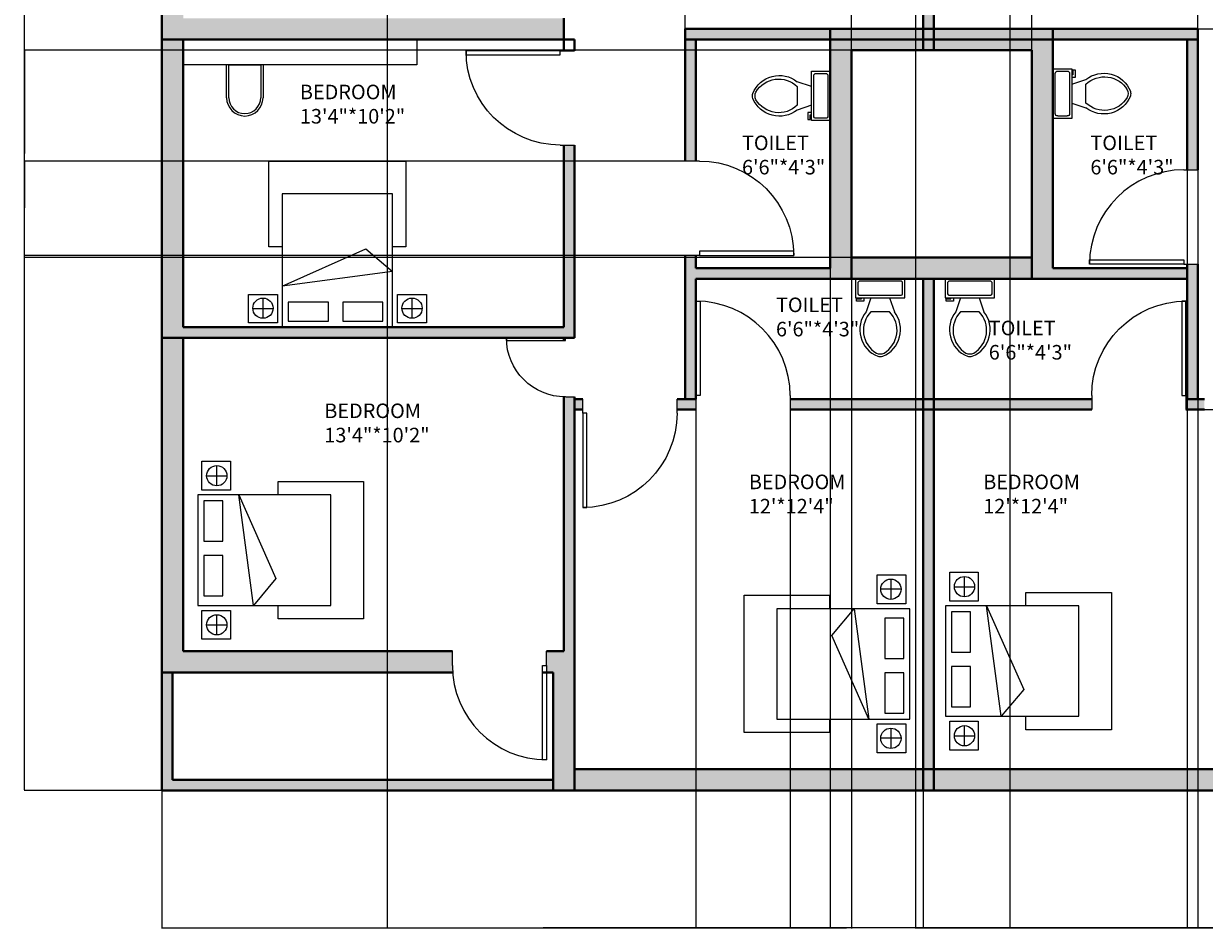
# Model space of a CAD drawing. Units: inches. Extents: x 1642 to 2399, y 1011 to 2291.
# Tile 1 of 7: x 1642 to 2143, y 1011 to 1395. Entities that reach past the tile are written whole.
import ezdxf

# ---------------------------------------------------------------- set-up
doc = ezdxf.new("R2010")
doc.units = ezdxf.units.IN
for name, color, linetype, lineweight in [('A-ANNO-DIMS', 2, 'Continuous', 18), ('A-AREA-IDEN', 7, 'Continuous', 20), ('A-DOOR', 4, 'Continuous', 25), ('A-FLOR-FIXT', 9, 'Continuous', 18), ('A-FURN', 8, 'Continuous', 18), ('A-WALL-PATT', 40, 'Continuous', 13), ('BED', 200, 'Continuous', 18), ('WALL', 40, 'Continuous', 40)]:
    doc.layers.add(name, color=color, linetype=linetype, lineweight=lineweight)
doc.styles.get("Standard").update_dxf_attribs({"font": 'arial.ttf'})
doc.dimstyles.get("Standard").update_dxf_attribs({"dimtxt": 0.18, "dimasz": 0.18, "dimexe": 0.18, "dimexo": 0.0625, "dimgap": 0.09, "dimtad": 0, "dimtih": 1, "dimtoh": 1, "dimdec": 4, "dimzin": 0, "dimdsep": 46, "dimtxsty": 'Standard', "dimcen": 0.09, "dimadec": 0, "dimazin": 0, "dimtfac": 1, "dimtdec": 4, "dimtofl": 0, "dimtmove": 0, "dimatfit": 3, "dimfxl": 1, "dimtolj": 1, "dimtzin": 0, "dimarcsym": 0})

# ---------------------------------------------------------------- blocks, each defined once
blk = doc.blocks.new('*U2')
for p, q in [((0, 0), (0, -6)), ((40, 0), (40, -6))]:
    blk.add_line(p, q)
blk.add_lwpolyline([(0, 0), (0, 40), (1.75, 40), (1.75, 0)], close=True)
blk.add_arc((0, 0), 40, 0, 90)
blk = doc.blocks.new('*U4')
for p, q in [((9.5, -6), (9.5, -2)), ((-10, -8.5), (-8, -8.5)), ((-10, -9.5), (-10, -8.5)), ((-7, -9.5), (-10, -9.5)), ((-8, -8.5), (-8, -8)), ((-7, -8), (-7, -9.5)), ((-4, -8), (-6, -14)), ((4, -8), (6, -14)), ((4, -14), (-4, -14))]:
    blk.add_line(p, q)
blk.add_lwpolyline([(10.5, -8), (10.5, 0), (-10.5, 0), (-10.5, -8)], close=True)
for points in [[(-9.5, -2), (-9.5, -6)], [(8.5, -1), (-8.5, -1)], [(-8.5, -7), (8.5, -7)]]:
    blk.add_lwpolyline(points)
for centre, radius, start, end in [((-8.62, -1.88), 0.884, 81.8699, 188.1301), ((8.62, -1.88), 0.884, 351.8699, 98.1301), ((-8.62, -6.12), 0.884, 171.8699, 278.1301), ((8.62, -6.12), 0.884, 261.8699, 8.1301), ((3.52, -21.58), 12.17, 141.4691, 247.9714), ((4.2, -21.82), 11.33, 136.3677, 238.9468), ((-3.52, -21.58), 12.17, 292.0284, 38.5307), ((-4.2, -21.82), 11.33, 301.053, 43.6321), ((0, -27.88), 4, 245.7318, 294.2682), ((0, -29), 4, 254.8605, 285.1395)]:
    blk.add_arc(centre, radius, start, end)
blk = doc.blocks.new('BED-DOUBLE-WITH-NIGHTSTANDS')
for p, q in [((8.62, 34.13), (8.62, 70.38)), ((8.62, 70.38), (66.79, 70.38)), ((66.79, 70.38), (66.79, 34.13)), ((14.22, 34.13), (8.62, 34.13)), ((14.22, 17.36), (49.69, 33.17)), ((49.69, 33.17), (61.11, 23.59)), ((66.79, 34.13), (61.11, 34.13)), ((61.11, 23.59), (14.22, 17.36)), ((6.17, 3.76), (6.17, 12.35)), ((69.41, 3.76), (69.41, 12.35)), ((1.82, 7.94), (10.42, 7.94)), ((65.06, 7.94), (73.65, 7.94))]:
    blk.add_line(p, q)
for points in [[(14.22, 0), (61.11, 0), (61.11, 56.52), (14.22, 56.52)], [(12.24, 1.79), (0, 1.79), (0, 13.82), (12.24, 13.82)], [(16.77, 2.51), (33.87, 2.51), (33.87, 10.66), (16.77, 10.66)], [(39.94, 2.51), (57.04, 2.51), (57.04, 10.66), (39.94, 10.66)], [(75.48, 1.79), (63.24, 1.79), (63.24, 13.82), (75.48, 13.82)]]:
    blk.add_lwpolyline(points, close=True)
for centre in [(6.12, 8.05), (69.36, 8.05)]:
    blk.add_circle(centre, 4.3)
blk = doc.blocks.new('DESK-WITH-CHAIR')
blk.add_lwpolyline([(0, 32.44), (99.14, 32.44), (99.14, 21.72), (0, 21.72)], close=True)
for points in [[(18.41, 7.73), (18.41, 21.72)], [(19.41, 7.73), (19.41, 21.72), (32.87, 21.72), (32.87, 7.73)], [(33.87, 21.72), (33.87, 7.73)]]:
    blk.add_lwpolyline(points)
for radius in [7.73, 6.73]:
    blk.add_arc((26.14, 7.73), radius, 180, 0)
blk = doc.blocks.new('*D33')
at = {"layer": 'A-ANNO-DIMS', "color": 0, "lineweight": -2, "transparency": 16777216}
for p, q in [((1700.65, 2232.46), (1642.19, 2232.46)), ((1642.37, 2232.28), (1642.37, 1651.26)), ((1642.37, 1069.89), (1642.37, 1650.9)), ((1700.65, 1069.71), (1642.19, 1069.71))]:
    blk.add_line(p, q, dxfattribs=at)
at = {"layer": 'A-ANNO-DIMS', "color": 0, "transparency": 16777216}
for points in [[(1642.34, 2232.28), (1642.4, 2232.28), (1642.37, 2232.46)], [(1642.34, 1069.89), (1642.4, 1069.89), (1642.37, 1069.71)]]:
    blk.add_solid(points, dxfattribs=at)
at = {"layer": 'Defpoints', "color": 0, "transparency": 16777216}
for p in [(1642.37, 2232.46), (1700.71, 2232.46), (1700.71, 1069.71)]:
    blk.add_point(p, dxfattribs=at)
at = {"layer": 'A-ANNO-DIMS', "color": 0, "transparency": 16777216, "insert": (1642.37, 1651.08), "char_height": 0.18, "attachment_point": 5}
blk.add_mtext('\\A1;1162.7', dxfattribs=at)
blk = doc.blocks.new('*D40')
at = {"layer": 'A-ANNO-DIMS', "color": 0, "lineweight": -2, "transparency": 16777216}
for p, q in [((1796.18, 1709.39), (1796.18, 1011.19)), ((2186.88, 1709.39), (2186.88, 1011.19)), ((1796.36, 1011.37), (1991.13, 1011.37)), ((2186.7, 1011.37), (1991.92, 1011.37))]:
    blk.add_line(p, q, dxfattribs=at)
at = {"layer": 'A-ANNO-DIMS', "color": 0, "transparency": 16777216}
for points in [[(1796.36, 1011.4), (1796.36, 1011.34), (1796.18, 1011.37)], [(2186.7, 1011.4), (2186.7, 1011.34), (2186.88, 1011.37)]]:
    blk.add_solid(points, dxfattribs=at)
at = {"layer": 'Defpoints', "color": 0, "transparency": 16777216}
for p in [(1796.18, 1709.46), (2186.88, 1709.46), (2186.88, 1011.37)]:
    blk.add_point(p, dxfattribs=at)
at = {"layer": 'A-ANNO-DIMS', "color": 0, "transparency": 16777216, "insert": (1991.53, 1011.37), "char_height": 0.18, "attachment_point": 5}
blk.add_mtext('\\A1;390.7', dxfattribs=at)
blk = doc.blocks.new('*D44')
at = {"layer": 'A-ANNO-DIMS', "color": 0, "lineweight": -2, "transparency": 16777216}
for p, q in [((1700.71, 1069.65), (1700.71, 1011.19)), ((2023.71, 1069.65), (2023.71, 1011.19)), ((1700.89, 1011.37), (1861.92, 1011.37)), ((2023.53, 1011.37), (1862.5, 1011.37))]:
    blk.add_line(p, q, dxfattribs=at)
at = {"layer": 'A-ANNO-DIMS', "color": 0, "transparency": 16777216}
for points in [[(1700.89, 1011.4), (1700.89, 1011.34), (1700.71, 1011.37)], [(2023.53, 1011.4), (2023.53, 1011.34), (2023.71, 1011.37)]]:
    blk.add_solid(points, dxfattribs=at)
at = {"layer": 'Defpoints', "color": 0, "transparency": 16777216}
for p in [(1700.71, 1069.71), (2023.71, 1069.71), (2023.71, 1011.37)]:
    blk.add_point(p, dxfattribs=at)
at = {"layer": 'A-ANNO-DIMS', "color": 0, "transparency": 16777216, "insert": (1862.21, 1011.37), "char_height": 0.18, "attachment_point": 5}
blk.add_mtext('\\A1;323', dxfattribs=at)
blk = doc.blocks.new('*D45')
at = {"layer": 'A-ANNO-DIMS', "color": 0, "lineweight": -2, "transparency": 16777216}
for p, q in [((2023.71, 1069.65), (2023.71, 1011.19)), ((2340.18, 1069.65), (2340.18, 1011.19)), ((2023.89, 1011.37), (2181.55, 1011.37)), ((2340, 1011.37), (2182.34, 1011.37))]:
    blk.add_line(p, q, dxfattribs=at)
at = {"layer": 'A-ANNO-DIMS', "color": 0, "transparency": 16777216}
for points in [[(2023.89, 1011.4), (2023.89, 1011.34), (2023.71, 1011.37)], [(2340, 1011.4), (2340, 1011.34), (2340.18, 1011.37)]]:
    blk.add_solid(points, dxfattribs=at)
at = {"layer": 'Defpoints', "color": 0, "transparency": 16777216}
for p in [(2023.71, 1069.71), (2340.18, 1069.71), (2340.18, 1011.37)]:
    blk.add_point(p, dxfattribs=at)
at = {"layer": 'A-ANNO-DIMS', "color": 0, "transparency": 16777216, "insert": (2181.95, 1011.37), "char_height": 0.18, "attachment_point": 5}
blk.add_mtext('\\A1;316.5', dxfattribs=at)
blk = doc.blocks.new('*D46')
at = {"layer": 'A-ANNO-DIMS', "color": 0, "lineweight": -2, "transparency": 16777216}
for p, q in [((2020.45, 1709.39), (2020.45, 1011.19)), ((2060.45, 1709.39), (2060.45, 1011.19)), ((2020.63, 1011.37), (2040.22, 1011.37)), ((2060.27, 1011.37), (2040.67, 1011.37))]:
    blk.add_line(p, q, dxfattribs=at)
at = {"layer": 'A-ANNO-DIMS', "color": 0, "transparency": 16777216}
for points in [[(2020.63, 1011.4), (2020.63, 1011.34), (2020.45, 1011.37)], [(2060.27, 1011.4), (2060.27, 1011.34), (2060.45, 1011.37)]]:
    blk.add_solid(points, dxfattribs=at)
at = {"layer": 'Defpoints', "color": 0, "transparency": 16777216}
for p in [(2020.45, 1709.46), (2060.45, 1709.46), (2060.45, 1011.37)]:
    blk.add_point(p, dxfattribs=at)
at = {"layer": 'A-ANNO-DIMS', "color": 0, "transparency": 16777216, "insert": (2040.45, 1011.37), "char_height": 0.18, "attachment_point": 5}
blk.add_mtext('\\A1;40', dxfattribs=at)
blk = doc.blocks.new('*D48')
at = {"layer": 'A-ANNO-DIMS', "color": 0, "lineweight": -2, "transparency": 16777216}
for p, q in [((1922.74, 1392.77), (1922.74, 2290.98)), ((1922.92, 2290.8), (2031.1, 2290.8)), ((2140.06, 2290.8), (2031.89, 2290.8)), ((2140.24, 1392.77), (2140.24, 2290.98))]:
    blk.add_line(p, q, dxfattribs=at)
at = {"layer": 'A-ANNO-DIMS', "color": 0, "transparency": 16777216}
for points in [[(1922.92, 2290.83), (1922.92, 2290.77), (1922.74, 2290.8)], [(2140.06, 2290.83), (2140.06, 2290.77), (2140.24, 2290.8)]]:
    blk.add_solid(points, dxfattribs=at)
at = {"layer": 'Defpoints', "color": 0, "transparency": 16777216}
for p in [(2140.24, 2290.8), (1922.74, 1392.71), (2140.24, 1392.71)]:
    blk.add_point(p, dxfattribs=at)
at = {"layer": 'A-ANNO-DIMS', "color": 0, "transparency": 16777216, "insert": (2031.49, 2290.8), "char_height": 0.18, "attachment_point": 5}
blk.add_mtext('\\A1;217.5', dxfattribs=at)
blk = doc.blocks.new('*D49')
at = {"layer": 'A-ANNO-DIMS', "color": 0, "lineweight": -2, "transparency": 16777216}
for p, q in [((2140.3, 1392.71), (2398.73, 1392.71)), ((2398.55, 1392.53), (2398.55, 1312.16)), ((2398.55, 1231.42), (2398.55, 1311.79)), ((2135.24, 1231.24), (2398.73, 1231.24))]:
    blk.add_line(p, q, dxfattribs=at)
at = {"layer": 'A-ANNO-DIMS', "color": 0, "transparency": 16777216}
for points in [[(2398.52, 1392.53), (2398.58, 1392.53), (2398.55, 1392.71)], [(2398.52, 1231.42), (2398.58, 1231.42), (2398.55, 1231.24)]]:
    blk.add_solid(points, dxfattribs=at)
at = {"layer": 'Defpoints', "color": 0, "transparency": 16777216}
for p in [(2140.24, 1392.71), (2135.18, 1231.24), (2398.55, 1231.24)]:
    blk.add_point(p, dxfattribs=at)
at = {"layer": 'A-ANNO-DIMS', "color": 0, "transparency": 16777216, "insert": (2398.55, 1311.98), "char_height": 0.18, "attachment_point": 5}
blk.add_mtext('\\A1;161.46', dxfattribs=at)
blk = doc.blocks.new('*D50')
at = {"layer": 'A-ANNO-DIMS', "color": 0, "lineweight": -2, "transparency": 16777216}
for p, q in [((1993.24, 1295.77), (1993.24, 2290.98)), ((1993.42, 2290.8), (2031.17, 2290.8)), ((2069.56, 2290.8), (2031.82, 2290.8)), ((2069.74, 1295.77), (2069.74, 2290.98))]:
    blk.add_line(p, q, dxfattribs=at)
at = {"layer": 'A-ANNO-DIMS', "color": 0, "transparency": 16777216}
for points in [[(1993.42, 2290.83), (1993.42, 2290.77), (1993.24, 2290.8)], [(2069.56, 2290.83), (2069.56, 2290.77), (2069.74, 2290.8)]]:
    blk.add_solid(points, dxfattribs=at)
at = {"layer": 'Defpoints', "color": 0, "transparency": 16777216}
for p in [(2069.74, 2290.8), (1993.24, 1295.71), (2069.74, 1295.71)]:
    blk.add_point(p, dxfattribs=at)
at = {"layer": 'A-ANNO-DIMS', "color": 0, "transparency": 16777216, "insert": (2031.49, 2290.8), "char_height": 0.18, "attachment_point": 5}
blk.add_mtext('\\A1;76.5', dxfattribs=at)
blk = doc.blocks.new('*D51')
at = {"layer": 'A-ANNO-DIMS', "color": 0, "lineweight": -2, "transparency": 16777216}
for p, q in [((2069.68, 1383.71), (1642.19, 1383.71)), ((1642.37, 1383.53), (1642.37, 1339.89)), ((1642.37, 1295.89), (1642.37, 1339.53)), ((2069.68, 1295.71), (1642.19, 1295.71))]:
    blk.add_line(p, q, dxfattribs=at)
at = {"layer": 'A-ANNO-DIMS', "color": 0, "transparency": 16777216}
for points in [[(1642.34, 1383.53), (1642.4, 1383.53), (1642.37, 1383.71)], [(1642.34, 1295.89), (1642.4, 1295.89), (1642.37, 1295.71)]]:
    blk.add_solid(points, dxfattribs=at)
at = {"layer": 'Defpoints', "color": 0, "transparency": 16777216}
for p in [(1642.37, 1383.71), (2069.74, 1383.71), (2069.74, 1295.71)]:
    blk.add_point(p, dxfattribs=at)
at = {"layer": 'A-ANNO-DIMS', "color": 0, "transparency": 16777216, "insert": (1642.37, 1339.71), "char_height": 0.18, "attachment_point": 5}
blk.add_mtext('\\A1;88', dxfattribs=at)
blk = doc.blocks.new('*D52')
at = {"layer": 'A-ANNO-DIMS', "color": 0, "lineweight": -2, "transparency": 16777216}
for p, q in [((1922.68, 1336.67), (1642.19, 1336.67)), ((1642.37, 1336.49), (1642.37, 1316.85)), ((1642.37, 1296.85), (1642.37, 1316.49)), ((1922.68, 1296.67), (1642.19, 1296.67))]:
    blk.add_line(p, q, dxfattribs=at)
at = {"layer": 'A-ANNO-DIMS', "color": 0, "transparency": 16777216}
for points in [[(1642.34, 1336.49), (1642.4, 1336.49), (1642.37, 1336.67)], [(1642.34, 1296.85), (1642.4, 1296.85), (1642.37, 1296.67)]]:
    blk.add_solid(points, dxfattribs=at)
at = {"layer": 'Defpoints', "color": 0, "transparency": 16777216}
for p in [(1642.37, 1336.67), (1922.74, 1336.67), (1922.74, 1296.67)]:
    blk.add_point(p, dxfattribs=at)
at = {"layer": 'A-ANNO-DIMS', "color": 0, "transparency": 16777216, "insert": (1642.37, 1316.67), "char_height": 0.18, "attachment_point": 5}
blk.add_mtext('\\A1;40', dxfattribs=at)
blk = doc.blocks.new('*D53')
at = {"layer": 'A-ANNO-DIMS', "color": 0, "lineweight": -2, "transparency": 16777216}
for p, q in [((1927.24, 1235.65), (1927.24, 1011.19)), ((1967.24, 1235.65), (1967.24, 1011.19)), ((1927.42, 1011.37), (1947.02, 1011.37)), ((1967.06, 1011.37), (1947.46, 1011.37))]:
    blk.add_line(p, q, dxfattribs=at)
at = {"layer": 'A-ANNO-DIMS', "color": 0, "transparency": 16777216}
for points in [[(1927.42, 1011.4), (1927.42, 1011.34), (1927.24, 1011.37)], [(1967.06, 1011.4), (1967.06, 1011.34), (1967.24, 1011.37)]]:
    blk.add_solid(points, dxfattribs=at)
at = {"layer": 'Defpoints', "color": 0, "transparency": 16777216}
for p in [(1927.24, 1235.71), (1967.24, 1235.71), (1967.24, 1011.37)]:
    blk.add_point(p, dxfattribs=at)
at = {"layer": 'A-ANNO-DIMS', "color": 0, "transparency": 16777216, "insert": (1947.24, 1011.37), "char_height": 0.18, "attachment_point": 5}
blk.add_mtext('\\A1;40', dxfattribs=at)
blk = doc.blocks.new('*D54')
at = {"layer": 'A-ANNO-DIMS', "color": 0, "lineweight": -2, "transparency": 16777216}
for p, q in [((1984.24, 1388.15), (1984.24, 1011.19)), ((1993.24, 1383.65), (1993.24, 1011.19)), ((1984.42, 1011.37), (1988.59, 1011.37)), ((1993.06, 1011.37), (1988.89, 1011.37))]:
    blk.add_line(p, q, dxfattribs=at)
at = {"layer": 'A-ANNO-DIMS', "color": 0, "transparency": 16777216}
for points in [[(1984.42, 1011.4), (1984.42, 1011.34), (1984.24, 1011.37)], [(1993.06, 1011.4), (1993.06, 1011.34), (1993.24, 1011.37)]]:
    blk.add_solid(points, dxfattribs=at)
at = {"layer": 'Defpoints', "color": 0, "transparency": 16777216}
for p in [(1984.24, 1388.21), (1993.24, 1383.71), (1993.24, 1011.37)]:
    blk.add_point(p, dxfattribs=at)
at = {"layer": 'A-ANNO-DIMS', "color": 0, "transparency": 16777216, "insert": (1988.74, 1011.37), "char_height": 0.18, "attachment_point": 5}
blk.add_mtext('\\A1;9', dxfattribs=at)
blk = doc.blocks.new('*D55')
at = {"layer": 'A-ANNO-DIMS', "color": 0, "lineweight": -2, "transparency": 16777216}
for p, q in [((2135.74, 1388.15), (2135.74, 1011.19)), ((2140.24, 1392.65), (2140.24, 1011.19)), ((2135.92, 1011.37), (2137.73, 1011.37)), ((2140.06, 1011.37), (2138.25, 1011.37))]:
    blk.add_line(p, q, dxfattribs=at)
at = {"layer": 'A-ANNO-DIMS', "color": 0, "transparency": 16777216}
for points in [[(2135.92, 1011.4), (2135.92, 1011.34), (2135.74, 1011.37)], [(2140.06, 1011.4), (2140.06, 1011.34), (2140.24, 1011.37)]]:
    blk.add_solid(points, dxfattribs=at)
at = {"layer": 'Defpoints', "color": 0, "transparency": 16777216}
for p in [(2135.74, 1388.21), (2140.24, 1392.71), (2140.24, 1011.37)]:
    blk.add_point(p, dxfattribs=at)
at = {"layer": 'A-ANNO-DIMS', "color": 0, "transparency": 16777216, "insert": (2137.99, 1011.37), "char_height": 0.18, "attachment_point": 5}
blk.add_mtext('\\A1;4.5', dxfattribs=at)

msp = doc.modelspace()

# ---------------------------------------------------------------- hatches: boundary and pattern name
at = {"layer": 'A-WALL-PATT'}
h = msp.add_hatch(color=256, dxfattribs=at)
h.dxf.hatch_style = 1
h.paths.add_polyline_path([(2340.1804, 2185.4562), (2211.0983, 2185.4562, -0.01876983), (2211.211, 2182.4562), (2211.211, 2176.4562), (2331.211, 2176.4562), (2331.211, 2043.4562), (2171.211, 2043.4562), (2171.211, 2038.9562), (2331.211, 2038.9562), (2331.211, 1916.9562), (2171.211, 1916.9562), (2171.211, 1918.9365), (2166.711, 1918.9365), (2166.711, 1912.4562), (2340.1804, 1912.4562)])
h.paths.add_polyline_path([(2171.211, 2043.4562), (2171.211, 2043.9025), (2170.5217, 2043.9025), (2166.711, 2043.9025), (2166.711, 2038.9562), (2166.711, 1958.9365), (2171.211, 1958.9365)], flags=17)
h.paths.add_polyline_path([(2129.211, 1971.5979), (2124.711, 1971.5979), (2124.711, 1918.4562), (2067.711, 1918.4562), (2067.711, 1913.9562), (2129.211, 1913.9562)])
h.paths.add_polyline_path([(2067.711, 2015.4562), (2124.711, 2015.4562), (2124.711, 2019.9562), (2058.711, 2019.9562), (2058.711, 2015.4562), (2058.711, 1922.9562), (1982.211, 1922.9562), (1982.211, 2015.4562), (1982.211, 2019.9562), (1916.211, 2019.9562), (1916.211, 2070.9562), (1911.711, 2070.9562), (1911.711, 2015.4562), (1911.711, 2012.302), (1916.211, 2012.302), (1916.211, 2015.4562), (1973.211, 2015.4562), (1973.211, 1918.4562), (1973.211, 1913.9562), (2017.1804, 1913.9562), (2067.711, 1913.9562), (2067.711, 1918.4562)])
h.paths.add_polyline_path([(2131.1386, 2075.4562), (2118.1934, 2075.4562), (2118.1934, 2070.9562), (2131.1386, 2070.9562)], flags=17)
h.paths.add_polyline_path([(1918.8034, 2075.4562), (1909.4956, 2075.4562), (1909.4956, 2070.9562), (1918.8034, 2070.9562)], flags=17)
h.paths.add_polyline_path([(1874.211, 2029.9562), (1869.711, 2029.9562), (1869.711, 1960.7404), (1874.211, 1960.7404)], flags=17)
h.paths.add_polyline_path([(1916.211, 1972.302), (1911.711, 1972.302), (1911.711, 1918.4562), (1916.211, 1918.4562)], flags=17)
h.paths.add_polyline_path([(2340.1804, 1912.4562), (2331.1804, 1912.4562), (2331.1804, 1794.4562), (2210.1804, 1794.4562), (2210.1804, 1789.9562), (2279.6804, 1789.9562), (2340.1804, 1789.9562)])
h.paths.add_polyline_path([(2288.6804, 1789.9562), (2279.6804, 1789.9562), (2279.6804, 1785.0846), (2285.6804, 1785.0846), (2288.6804, 1785.0846)], flags=17)
h.paths.add_polyline_path([(2169.6804, 1789.9562), (2170.1804, 1789.9562), (2170.1804, 1794.4562), (2165.1804, 1794.4562), (2165.1804, 1713.9562), (2165.1804, 1709.4562), (2279.6804, 1709.4562), (2279.6804, 1718.4562), (2169.6804, 1718.4562)])
h.paths.add_polyline_path([(2288.6804, 1745.1973, -0.01876983), (2285.6804, 1745.0846), (2279.6804, 1745.0846), (2279.6804, 1709.4562), (2340.1804, 1709.4562), (2340.1804, 1789.9562), (2335.6804, 1789.9562), (2335.6804, 1713.9562), (2288.6804, 1713.9562)])
h.paths.add_polyline_path([(2165.1804, 1713.9562), (2140.6229, 1713.9562), (2088.923, 1713.9562), (2069.7509, 1713.9562), (2060.4457, 1713.9562), (2060.4457, 1709.4562), (2165.1804, 1709.4562)])
h.paths.add_polyline_path([(2020.4457, 1713.9562), (2017.1804, 1713.9562), (2012.6804, 1713.9562), (2009.1946, 1713.9562), (2009.1946, 1709.4562), (2020.4457, 1709.4562)])
h.paths.add_polyline_path([(1969.1946, 1713.9562), (1864.6804, 1713.9562), (1864.6804, 1798.9562), (1860.1804, 1798.9562), (1860.1804, 1792.9562), (1860.1804, 1752.9562), (1860.1804, 1718.4562), (1750.1804, 1718.4562), (1750.1804, 1749.2419), (1744.1804, 1749.2419, -0.01876983), (1741.1804, 1749.3546), (1741.1804, 1709.4562), (1969.1946, 1709.4562)])
h.paths.add_polyline_path([(1741.1804, 1803.4562), (1700.711, 1803.4562), (1700.711, 1794.4562), (1741.1804, 1794.4562)])
h.paths.add_polyline_path([(1820.1804, 1798.9562), (1741.1804, 1798.9562), (1741.1804, 1794.4562), (1741.1804, 1790.0365), (1741.1804, 1789.2419), (1744.1804, 1789.2419), (1750.1804, 1789.2419), (1750.1804, 1794.4562), (1820.1804, 1794.4562)], flags=17)
h.paths.add_polyline_path([(1800.6804, 1709.4562), (1796.1804, 1709.4562), (1796.1804, 1592.7078), (1978.9325, 1592.7078), (1978.9325, 1597.2078), (1800.6804, 1597.2078)])
h.paths.add_polyline_path([(2097.0678, 1709.4562), (2088.0678, 1709.4562), (2088.0678, 1599.6874), (2088.0678, 1597.2078), (2097.0678, 1597.2078)], flags=17)
h.paths.add_polyline_path([(2186.8766, 1709.4562), (2182.3766, 1709.4562), (2182.3766, 1597.2078), (2071.4624, 1597.2078), (2071.4624, 1592.7078), (2186.8766, 1592.7078)])
h.paths.add_polyline_path([(2078.1934, 2075.4562), (2022.711, 2075.4562), (2022.711, 2223.4562), (2166.711, 2223.4562), (2166.711, 2075.4562), (2166.711, 2070.9562), (2171.211, 2070.9562), (2171.211, 2138.8919), (2171.211, 2227.9562), (2335.711, 2227.9562), (2335.711, 2185.4562), (2340.1804, 2185.4562), (2340.1804, 2232.4562), (1874.211, 2232.4562), (1874.211, 2223.4562), (2018.211, 2223.4562), (2018.211, 2075.4562), (1958.8034, 2075.4562), (1958.8034, 2070.9562), (2018.211, 2070.9562), (2018.211, 2019.9562), (1982.211, 2019.9562), (1982.211, 2015.4562), (1982.211, 2010.9562), (2058.711, 2010.9562), (2058.711, 2015.4562), (2058.711, 2019.9562), (2022.711, 2019.9562), (2022.711, 2070.9562), (2078.1934, 2070.9562)])
h.paths.add_polyline_path([(1874.211, 2171.9562), (1874.211, 2176.4562), (1861.9371, 2176.4562), (1861.9371, 2173.4562), (1861.9371, 2167.4562), (1869.711, 2167.4562), (1869.711, 2069.7602), (1874.211, 2069.7602)], flags=17)
h.paths.add_polyline_path([(1705.211, 2227.9562), (1865.211, 2227.9562), (1865.211, 2176.4562), (1874.211, 2176.4562), (1874.211, 2232.4562), (1700.711, 2232.4562), (1700.711, 2176.4562), (1705.211, 2176.4562)])
h.paths.add_polyline_path([(1709.711, 2167.4562), (1821.9371, 2167.4562), (1821.9371, 2173.4562, -0.01876983), (1822.0498, 2176.4562), (1700.711, 2176.4562), (1700.711, 1913.9562), (1860.1804, 1913.9562), (1864.6804, 1913.9562), (1973.211, 1913.9562), (1973.211, 1918.4562), (1916.211, 1918.4562), (1874.211, 1918.4562), (1874.211, 1920.7404), (1869.711, 1920.7404), (1869.711, 1918.4562), (1860.1804, 1918.4562), (1709.711, 1918.4562), (1709.711, 2029.9562), (1874.211, 2029.9562), (1874.211, 2037.0364), (1869.711, 2037.0364), (1869.711, 2034.4562), (1709.711, 2034.4562)])
h.paths.add_polyline_path([(2017.1804, 1913.9562), (2012.6804, 1913.9562), (2012.6804, 1713.9562), (2017.1804, 1713.9562)])
h.paths.add_polyline_path([(1952.4341, 2110.3716), (2000.4134, 2110.3716), (2000.4134, 2133.4189), (1952.4341, 2133.4189)], flags=25)
h.paths.add_polyline_path([(2042.3983, 2110.7121), (2090.3775, 2110.7121), (2090.3775, 2133.7594), (2042.3983, 2133.7594)], flags=25)
h.paths.add_polyline_path([(2201.7332, 2091.8715), (2249.7125, 2091.8715), (2249.7125, 2114.9188), (2201.7332, 2114.9188)], flags=25)
h.paths.add_polyline_path([(1805.186, 2077.6915), (1853.1653, 2077.6915), (1853.1653, 2100.7388), (1805.186, 2100.7388)], flags=25)
h.paths.add_polyline_path([(1794.8897, 1974.6584), (1842.869, 1974.6584), (1842.869, 1997.7057), (1794.8897, 1997.7057)], flags=25)
h.paths.add_polyline_path([(2229.1796, 2204.4209), (2315.1362, 2204.4209), (2315.1362, 2217.1488), (2229.1796, 2217.1488)], flags=25)
h.paths.add_polyline_path([(1715.2159, 2199.5328), (1801.1724, 2199.5328), (1801.1724, 2212.2607), (1715.2159, 2212.2607)], flags=25)
h.paths.add_polyline_path([(2230.7681, 1755.7109), (2271.7283, 1755.7109), (2271.7283, 1778.7582), (2230.7681, 1778.7582)], flags=25)
h.paths.add_polyline_path([(1763.4713, 1764.1742), (1804.4315, 1764.1742), (1804.4315, 1787.2215), (1763.4713, 1787.2215)], flags=25)
h.paths.add_polyline_path([(2076.2643, 1955.0495), (2111.326, 1955.0495), (2111.326, 1978.0968), (2076.2643, 1978.0968)], flags=25)
h.paths.add_polyline_path([(1932.854, 1956.1217), (1967.9158, 1956.1217), (1967.9158, 1979.169), (1932.854, 1979.169)], flags=25)
h.paths.add_polyline_path([(2048.1203, 2031.6107), (2083.1821, 2031.6107), (2083.1821, 2054.658), (2048.1203, 2054.658)], flags=25)
h.paths.add_polyline_path([(2163.5754, 1863.7569), (2208.2347, 1863.7569), (2208.2347, 1886.8042), (2163.5754, 1886.8042)], flags=9)
h.paths.add_polyline_path([(2039.9286, 1809.0957), (2084.5879, 1809.0957), (2084.5879, 1832.143), (2039.9286, 1832.143)], flags=9)
h.paths.add_polyline_path([(1901.0045, 1814.0452), (1945.6638, 1814.0452), (1945.6638, 1837.0925), (1901.0045, 1837.0925)], flags=9)
h.paths.add_polyline_path([(1833.7282, 1852.5627), (1878.3875, 1852.5627), (1878.3875, 1875.61), (1833.7282, 1875.61)], flags=9)
h.paths.add_polyline_path([(2219.1375, 1926.2139), (2267.1167, 1926.2139), (2267.1167, 1949.2612), (2219.1375, 1949.2612)], flags=25)
h.paths.add_polyline_path([(1956.9598, 2029.7735), (1992.0216, 2029.7735), (1992.0216, 2052.8208), (1956.9598, 2052.8208)], flags=25)
h.paths.add_polyline_path([(2229.3, 1523.3399), (2270.2602, 1523.3399), (2270.2602, 1546.3872), (2229.3, 1546.3872)], flags=9)
h.paths.add_polyline_path([(1772.3039, 1526.9922), (1813.2641, 1526.9922), (1813.2641, 1550.0394), (1772.3039, 1550.0394)], flags=9)
h.paths.add_polyline_path([(2172.587, 1420.6999), (2217.2463, 1420.6999), (2217.2463, 1443.7472), (2172.587, 1443.7472)], flags=9)
h.paths.add_polyline_path([(1814.3549, 1422.215), (1859.0143, 1422.215), (1859.0143, 1445.2623), (1814.3549, 1445.2623)], flags=9)
h.paths.add_polyline_path([(2186.0372, 1305.6227), (2234.0165, 1305.6227), (2234.0165, 1328.67), (2186.0372, 1328.67)], flags=9)
h.paths.add_polyline_path([(1756.747, 1349.0694), (1804.7263, 1349.0694), (1804.7263, 1372.1167), (1756.747, 1372.1167)], flags=9)
h.paths.add_polyline_path([(2239.449, 1214.6184), (2287.4282, 1214.6184), (2287.4282, 1237.6657), (2239.449, 1237.6657)], flags=9)
h.paths.add_polyline_path([(1767.104, 1213.8348), (1815.0832, 1213.8348), (1815.0832, 1236.8821), (1767.104, 1236.8821)], flags=9)
h.paths.add_polyline_path([(2046.6809, 1183.6854), (2094.6602, 1183.6854), (2094.6602, 1206.7327), (2046.6809, 1206.7327)], flags=9)
h.paths.add_polyline_path([(1947.2155, 1183.6854), (1995.1948, 1183.6854), (1995.1948, 1206.7327), (1947.2155, 1206.7327)], flags=9)
h.paths.add_polyline_path([(1959.3556, 1258.7871), (1994.4174, 1258.7871), (1994.4174, 1281.8344), (1959.3556, 1281.8344)], flags=9)
h.paths.add_polyline_path([(2049.6419, 1248.9629), (2084.7036, 1248.9629), (2084.7036, 1272.0102), (2049.6419, 1272.0102)], flags=9)
h.paths.add_polyline_path([(2092.7532, 1327.4852), (2127.815, 1327.4852), (2127.815, 1350.5325), (2092.7532, 1350.5325)], flags=9)
h.paths.add_polyline_path([(1944.9358, 1327.4852), (1979.9976, 1327.4852), (1979.9976, 1350.5325), (1944.9358, 1350.5325)], flags=9)
h.paths.add_polyline_path([(1974.5055, 1650.063), (2006.3695, 1650.063), (2006.3695, 1662.7909), (1974.5055, 1662.7909)], flags=9)
h = msp.add_hatch(color=256, dxfattribs=at)
h.dxf.hatch_style = 1
h.paths.add_polyline_path([(2078.7415, 1388.2078), (2028.211, 1388.2078), (2028.211, 1383.7078), (2069.7415, 1383.7078), (2069.7415, 1291.2078), (2069.7415, 1286.7078), (2135.7415, 1286.7078), (2135.7415, 1291.2078), (2078.7415, 1291.2078)])
h.paths.add_polyline_path([(1993.2415, 1383.7078), (2023.711, 1383.7078), (2023.711, 1388.2078), (1984.2415, 1388.2078), (1984.2415, 1291.2078), (1927.2415, 1291.2078), (1927.2415, 1296.6705), (1922.7415, 1296.6705), (1922.7415, 1291.2078), (1922.7415, 1235.7078), (1927.2415, 1235.7078), (1927.2415, 1237.2428), (1927.2415, 1277.2428), (1927.2415, 1286.7078), (1993.2415, 1286.7078), (1993.2415, 1291.2078)])
h.paths.add_polyline_path([(1927.2415, 1388.2078), (1922.7415, 1388.2078), (1922.7415, 1336.6705), (1927.2415, 1336.6705)])
h.paths.add_polyline_path([(1984.2415, 1392.7078), (1922.7415, 1392.7078), (1922.7415, 1388.2078), (1984.2415, 1388.2078)])
h.paths.add_polyline_path([(2023.711, 1392.7078), (1984.2415, 1392.7078), (1984.2415, 1388.2078), (2023.711, 1388.2078)])
h.paths.add_polyline_path([(2078.7415, 1392.7078), (2028.211, 1392.7078), (2028.211, 1388.2078), (2078.7415, 1388.2078)])
h.paths.add_polyline_path([(2140.2415, 1392.7078), (2078.7415, 1392.7078), (2078.7415, 1388.2078), (2135.7415, 1388.2078), (2140.2415, 1388.2078)])
h.paths.add_polyline_path([(2028.211, 1592.7078), (2023.711, 1592.7078), (2023.711, 1392.7078), (2028.211, 1392.7078)])
h.paths.add_polyline_path([(2028.211, 1388.2078), (2023.711, 1388.2078), (2023.711, 1383.7078), (2028.211, 1383.7078)])
h.paths.add_polyline_path([(2028.211, 1392.7078), (2023.711, 1392.7078), (2023.711, 1388.2078), (2028.211, 1388.2078)])
h.paths.add_polyline_path([(2140.2415, 1388.2078), (2135.7415, 1388.2078), (2135.7415, 1332.9578), (2140.2415, 1332.9578)])
h.paths.add_polyline_path([(2069.7415, 1291.2078), (2069.7415, 1295.7078), (2028.211, 1295.7078), (2023.711, 1295.7078), (1993.2415, 1295.7078), (1993.2415, 1291.2078), (1993.2415, 1286.7078), (2029.2415, 1286.7078), (2047.9002, 1286.7078), (2053.9738, 1286.7078), (2069.7415, 1286.7078)])
h.paths.add_polyline_path([(2140.2415, 1291.2078), (2140.2415, 1292.9578), (2135.7415, 1292.9578), (2135.7415, 1269.1323), (2135.7415, 1235.7078), (2140.2415, 1235.7078)])
h.paths.add_polyline_path([(2232.0378, 1392.7078), (2164.6804, 1392.7078), (2164.6804, 1388.2078), (2232.0378, 1388.2078)])
h.paths.add_polyline_path([(2331.1804, 1392.7078), (2232.0378, 1392.7078), (2232.0378, 1388.2078), (2331.1804, 1388.2078)])
h.paths.add_polyline_path([(2340.1804, 1392.7078), (2331.1804, 1392.7078), (2331.1804, 1388.2078), (2340.1804, 1388.2078)])
h.paths.add_polyline_path([(2340.1804, 1388.2078), (2331.1804, 1388.2078), (2331.1804, 1381.9887), (2331.1804, 1266.2078), (2340.1804, 1266.2078)])
h.paths.add_polyline_path([(2331.1804, 1266.2078), (2169.1804, 1266.2078), (2169.1804, 1342.6266), (2164.6804, 1342.6266), (2164.6804, 1266.2078), (2164.6804, 1261.6393), (2168.4442, 1261.6393), (2169.1804, 1261.6393), (2169.1804, 1261.7078), (2331.1804, 1261.7078)])
h.paths.add_polyline_path([(2340.1804, 1266.2078), (2331.1804, 1266.2078), (2331.1804, 1261.7078), (2340.1804, 1261.7078)])
h.paths.add_polyline_path([(2340.1804, 1503.2078), (2331.1804, 1503.2078), (2331.1804, 1392.7078), (2340.1804, 1392.7078)])
h.paths.add_polyline_path([(2340.1804, 1261.7078), (2331.1804, 1261.7078), (2331.1804, 1139.2078), (2331.0462, 1128.7078), (2340.1804, 1128.7078)])
h.paths.add_polyline_path([(2169.1804, 1236.5578, -0.00733557), (2168.4442, 1236.547), (2164.6804, 1236.547), (2164.6804, 1128.7078), (2169.1804, 1128.7078)])
h.paths.add_polyline_path([(2095.1813, 1235.7078), (2028.211, 1235.7078), (2028.211, 1231.2428), (2095.1813, 1231.2428)])
h.paths.add_polyline_path([(2028.211, 1286.7078), (2023.711, 1286.7078), (2023.711, 1235.7078), (2028.211, 1235.7078)])
h.paths.add_polyline_path([(2028.211, 1235.7078), (2023.711, 1235.7078), (2023.711, 1231.2428), (2028.211, 1231.2428)])
h.paths.add_polyline_path([(2023.711, 1235.7078), (1967.2415, 1235.7078), (1967.2415, 1231.2428), (2023.711, 1231.2428)])
h.paths.add_polyline_path([(2028.211, 1231.2428), (2023.711, 1231.2428), (2023.711, 1078.7078), (2028.211, 1078.7078)])
h.paths.add_polyline_path([(1866.711, 1074.2078), (1705.211, 1074.2078), (1705.211, 1119.7078), (1700.711, 1119.7078), (1700.711, 1069.7078), (1866.711, 1069.7078)])
h.paths.add_polyline_path([(2023.711, 1078.7078), (1875.711, 1078.7078), (1875.711, 1074.2078), (1875.711, 1069.7078), (2023.711, 1069.7078)])
h.paths.add_polyline_path([(2028.211, 1078.7078), (2023.711, 1078.7078), (2023.711, 1069.7078), (2028.211, 1069.7078)])
h.paths.add_polyline_path([(2164.6804, 1078.7078), (2028.211, 1078.7078), (2028.211, 1069.7078), (2164.6804, 1069.7078), (2164.6804, 1074.2078)])
h = msp.add_hatch(color=256, dxfattribs=at)
h.dxf.hatch_style = 1
h.paths.add_polyline_path([(1875.711, 1343.4643), (1871.211, 1343.4643), (1871.211, 1266.2078), (1709.711, 1266.2078), (1709.711, 1388.2078), (1700.711, 1388.2078), (1700.711, 1261.7078), (1709.711, 1261.7078), (1875.711, 1261.7078)])
h.paths.add_polyline_path([(1761.211, 1583.7078), (1761.211, 1588.2078), (1761.211, 1592.7078), (1700.711, 1592.7078), (1700.711, 1388.2078), (1709.711, 1388.2078), (1808.8535, 1388.2078), (1871.211, 1388.2078), (1871.211, 1397.2078), (1709.711, 1397.2078), (1709.711, 1503.2078), (1761.211, 1503.2078), (1825.4443, 1503.2078), (1825.4443, 1507.7078), (1761.211, 1507.7078), (1705.211, 1507.7078), (1705.211, 1516.7078), (1705.211, 1588.2078), (1752.211, 1588.2078), (1752.211, 1516.7078), (1752.211, 1507.7078), (1761.211, 1507.7078)])
h.paths.add_polyline_path([(1875.711, 1592.7078), (1761.211, 1592.7078), (1761.211, 1588.2078), (1761.211, 1583.7078), (1871.211, 1583.7078), (1871.211, 1507.7078), (1871.211, 1503.2078), (1875.711, 1503.2078), (1875.711, 1551.7879), (1875.711, 1583.7078)])
h.paths.add_polyline_path([(1823.9074, 1128.7078), (1709.711, 1128.7078), (1709.711, 1261.7078), (1700.711, 1261.7078), (1700.711, 1119.7078), (1705.211, 1119.7078), (1709.711, 1119.7078), (1824.02, 1119.7078, -0.01876983), (1823.9074, 1122.7078)])
h.paths.add_polyline_path([(1875.711, 1236.6154), (1871.9471, 1236.6154, -0.00733557), (1871.211, 1236.6262), (1871.211, 1128.7078), (1863.9074, 1128.7078), (1863.9074, 1122.7078), (1863.9074, 1119.7078), (1866.711, 1119.7078), (1866.711, 1074.2078), (1866.711, 1069.7078), (1875.711, 1069.7078), (1875.711, 1074.2078), (1875.711, 1128.7078)])
h.paths.add_polyline_path([(2173.6804, 1119.7078), (2176.9153, 1119.7078), (2176.9153, 1122.7078), (2176.9153, 1128.7078), (2164.6804, 1128.7078), (2164.6804, 1074.2078), (2164.6804, 1069.7078), (2340.1804, 1069.7078), (2340.1804, 1074.2078), (2335.6804, 1074.2078), (2180.1804, 1074.2078), (2173.6804, 1074.2078)])
h.paths.add_polyline_path([(2340.1804, 1128.7078), (2216.9153, 1128.7078), (2216.9153, 1122.7078, -0.01876983), (2216.8027, 1119.7078), (2340.1804, 1119.7078)], flags=17)
h.paths.add_polyline_path([(2340.1804, 1119.7078), (2335.6804, 1119.7078), (2335.6804, 1074.2078), (2340.1804, 1074.2078)], flags=17)
h.paths.add_polyline_path([(2169.1804, 1592.7078), (2164.6804, 1592.7078), (2164.6804, 1507.7078), (2169.1804, 1507.7078)])
h.paths.add_polyline_path([(2340.1804, 1592.7078), (2169.1804, 1592.7078), (2169.1804, 1588.2078), (2340.1804, 1588.2078)])
h.paths.add_polyline_path([(2340.1804, 1507.7078), (2212.6763, 1507.7078), (2212.6763, 1503.2078), (2340.1804, 1503.2078)])
h.paths.add_polyline_path([(2290.8982, 1588.2078), (2286.3982, 1588.2078), (2286.3982, 1549.1888), (2290.8982, 1549.1888)])
h = msp.add_hatch(color=256, dxfattribs=at)
h.dxf.hatch_style = 1
h.paths.add_polyline_path([(1871.211, 1507.7078), (1865.4443, 1507.7078), (1865.4443, 1503.2078), (1871.211, 1503.2078)])
h.paths.add_polyline_path([(2172.6763, 1507.7078), (2164.6804, 1507.7078), (2164.6804, 1504.0795), (2164.6804, 1503.2078), (2172.6763, 1503.2078)])
h.paths.add_polyline_path([(2290.8982, 1509.1888), (2286.3982, 1509.1888), (2286.3982, 1507.7078), (2290.8982, 1507.7078)])
h.paths.add_polyline_path([(2169.1804, 1388.2078), (2164.6804, 1388.2078), (2164.6804, 1382.6266), (2169.1804, 1382.6266)])
h.paths.add_polyline_path([(2142.989, 1235.7078), (2135.7415, 1235.7078), (2135.1813, 1235.7078), (2135.1813, 1231.2428), (2143.0228, 1231.2428, -0.01396842), (2142.989, 1232.4541)])
h.paths.add_polyline_path([(1927.2415, 1235.7078), (1919.2515, 1235.7078), (1919.2515, 1231.2428), (1926.6813, 1231.2428), (1927.2415, 1231.2428)])
h.paths.add_polyline_path([(1879.2515, 1235.7078), (1875.711, 1235.7078), (1875.711, 1231.2428), (1879.2515, 1231.2428)])

# ---------------------------------------------------------------- linework, layer by layer
at = {"layer": 'WALL'}
for p, q in [((2023.711, 1592.7078), (2023.711, 1392.7078)), ((2023.711, 1592.7078), (2023.711, 1392.7078)), ((2028.211, 1592.7078), (2028.211, 1388.2078)), ((2028.211, 1592.7078), (2028.211, 1392.7078)), ((1871.211, 1388.2078), (1871.211, 1397.2078)), ((1709.711, 1388.2078), (1700.711, 1388.2078)), ((1700.711, 1388.2078), (1709.711, 1388.2078)), ((1871.211, 1388.2078), (1709.711, 1388.2078)), ((1709.711, 1388.2078), (1709.711, 1266.2078)), ((1871.211, 1388.2078), (1871.211, 1383.4643)), ((1875.711, 1388.2078), (1871.211, 1388.2078)), ((1875.711, 1388.2078), (1875.711, 1383.4643)), ((2023.711, 1392.7078), (1922.7415, 1392.7078)), ((1922.7415, 1392.7078), (2028.211, 1392.7078)), ((1922.7415, 1388.2078), (1922.7415, 1392.7078)), ((2028.211, 1388.2078), (1922.7415, 1388.2078)), ((1984.2415, 1388.2078), (1922.7415, 1388.2078)), ((1922.7415, 1336.6705), (1922.7415, 1388.2078)), ((1927.2415, 1388.2078), (1984.2415, 1388.2078)), ((1927.2415, 1336.6705), (1927.2415, 1388.2078)), ((1984.2415, 1388.2078), (1984.2415, 1392.7078)), ((1984.2415, 1388.2078), (1984.2415, 1291.2078)), ((2023.711, 1392.7078), (2140.2415, 1392.7078)), ((2023.711, 1392.7078), (2023.711, 1383.7078)), ((2023.711, 1392.7078), (2140.2415, 1392.7078)), ((2028.211, 1388.2078), (2140.2415, 1388.2078)), ((2028.211, 1388.2078), (2028.211, 1383.7078)), ((2078.7415, 1388.2078), (2078.7415, 1392.7078)), ((2078.7415, 1388.2078), (2135.7415, 1388.2078)), ((2135.7415, 1388.2078), (2078.7415, 1388.2078)), ((2078.7415, 1388.2078), (2078.7415, 1291.2078)), ((2135.7415, 1388.2078), (2135.7415, 1332.9578)), ((2140.2415, 1332.9578), (2140.2415, 1392.7078)), ((1993.2415, 1383.7078), (1993.2415, 1291.2078)), ((1993.2415, 1383.7078), (2069.7415, 1383.7078)), ((2069.7415, 1383.7078), (2069.7415, 1291.2078)), ((1871.211, 1343.4643), (1871.211, 1266.2078)), ((1875.711, 1343.4643), (1875.711, 1261.7078)), ((1922.7415, 1291.2078), (1922.7415, 1296.6705)), ((1927.2415, 1291.2078), (1927.2415, 1296.6705)), ((1993.2415, 1295.7078), (2023.711, 1295.7078)), ((2023.711, 1295.7078), (2037.2251, 1295.7078)), ((2028.211, 1295.7078), (2069.7415, 1295.7078)), ((2135.7415, 1292.9578), (2135.7415, 1269.1323)), ((2140.2415, 1291.2078), (2140.2415, 1292.9578)), ((1922.7415, 1235.7078), (1922.7415, 1291.2078)), ((1927.2415, 1291.2078), (1984.2415, 1291.2078)), ((1993.2415, 1291.2078), (1993.2415, 1286.7078)), ((2069.7415, 1291.2078), (2069.7415, 1286.7078)), ((2078.7415, 1291.2078), (2135.7415, 1291.2078)), ((2140.2415, 1291.2078), (2140.2415, 1235.7078)), ((1927.2415, 1235.7078), (1927.2415, 1286.7078)), ((1927.2415, 1286.7078), (2029.2415, 1286.7078)), ((2023.711, 1286.7078), (2023.711, 1069.7078)), ((2028.211, 1286.7078), (2028.211, 1069.7078)), ((2029.2415, 1286.7078), (2047.9002, 1286.7078)), ((2033.7415, 1286.7078), (2135.7415, 1286.7078)), ((2135.7415, 1286.7078), (2135.7415, 1235.7078)), ((1709.711, 1266.2078), (1871.211, 1266.2078)), ((1709.711, 1261.7078), (1700.711, 1261.7078)), ((1709.711, 1261.7078), (1875.711, 1261.7078)), ((1709.711, 1261.7078), (1709.711, 1128.7078)), ((1871.211, 1261.7078), (1871.211, 1260.61)), ((1871.211, 1236.6262), (1871.211, 1128.7078)), ((1875.711, 1236.6154), (1875.711, 1119.7078)), ((1879.2515, 1235.7078), (1875.711, 1235.7078)), ((1927.2415, 1235.7078), (1919.2515, 1235.7078)), ((1967.2415, 1235.7078), (2095.1813, 1235.7078)), ((2135.1813, 1235.7078), (2135.7415, 1235.7078)), ((2135.7415, 1235.7078), (2142.989, 1235.7078)), ((1879.2515, 1231.2428), (1875.711, 1231.2428)), ((1926.6813, 1231.2428), (1919.2515, 1231.2428)), ((1926.6813, 1231.2428), (1927.2415, 1231.2428)), ((1967.2415, 1231.2428), (2095.1813, 1231.2428)), ((2135.1813, 1231.2428), (2143.0228, 1231.2428)), ((1709.711, 1128.7078), (1823.9074, 1128.7078)), ((1863.9074, 1128.7078), (1871.211, 1128.7078)), ((1875.711, 1074.2078), (1875.711, 1128.7078)), ((1709.711, 1119.7078), (1700.711, 1119.7078)), ((1700.711, 1119.7078), (1705.211, 1119.7078)), ((1705.211, 1119.7078), (1705.211, 1074.2078)), ((1709.711, 1119.7078), (1824.02, 1119.7078)), ((1862.1574, 1119.7078), (1866.711, 1119.7078)), ((1866.711, 1074.2078), (1866.711, 1119.7078)), ((1875.711, 1078.7078), (2164.6804, 1078.7078)), ((1700.711, 1069.7078), (1700.711, 1074.2078)), ((1705.211, 1074.2078), (1866.711, 1074.2078)), ((1866.711, 1074.2078), (1866.711, 1069.7078)), ((1875.711, 1074.2078), (1875.711, 1069.7078)), ((1875.711, 1069.7078), (2164.6804, 1069.7078))]:
    msp.add_line(p, q, dxfattribs=at)
msp.add_lwpolyline([(2071.4624, 1592.7078), (2340.1804, 1592.7078), (2340.1804, 1069.7078), (1700.711, 1069.7078), (1700.711, 1592.7078), (1978.9325, 1592.7078)], dxfattribs=at)

# ---------------------------------------------------------------- block references
at = {"layer": 'A-DOOR', "xscale": -1}
for p, rotation in [((1869.711, 1383.4643), 90), ((1928.7415, 1296.6705), 270), ((1879.2515, 1229.7078), 180)]:
    msp.add_blockref('*U2', p, dxfattribs=dict(at, rotation=rotation))
at = {"layer": 'A-DOOR'}
for p, rotation in [((2134.2415, 1292.9578), 90), ((1863.9074, 1122.7078), 180)]:
    msp.add_blockref('*U2', p, dxfattribs=dict(at, rotation=rotation))
msp.add_blockref('*U2', (1927.2415, 1237.2428), dxfattribs=at)
at = {"layer": 'A-DOOR', "xscale": -1}
msp.add_blockref('*U2', (2135.1813, 1237.2428), dxfattribs=at)
at = {"layer": 'A-DOOR', "xscale": -0.6273086553554587, "yscale": 0.6273086553554587, "zscale": 0.6273086553554587, "rotation": 90}
msp.add_blockref('*U2', (1871.9471, 1261.7078), dxfattribs=at)
at = {"layer": 'A-FLOR-FIXT', "xscale": -1}
for p, rotation in [((1984.2415, 1364.3075), 270), ((2078.7415, 1365.2728), 90)]:
    msp.add_blockref('*U4', p, dxfattribs=dict(at, rotation=rotation))
at = {"layer": 'A-FLOR-FIXT'}
for p in [(2005.4444, 1286.7078), (2043.4738, 1286.7078)]:
    msp.add_blockref('*U4', p, dxfattribs=at)
at = {"layer": 'A-FURN'}
msp.add_blockref('DESK-WITH-CHAIR', (1709.711, 1355.7723), dxfattribs=at)
at = {"layer": 'BED'}
msp.add_blockref('BED-DOUBLE-WITH-NIGHTSTANDS', (1737.4395, 1266.2078), dxfattribs=at)
for p, rotation in [((1715.8905, 1209.3127), 270.0000000000011), ((2018.0361, 1085.6786), 90.00000000000033), ((2033.1568, 1162.2521), 270.0000000000003)]:
    msp.add_blockref('BED-DOUBLE-WITH-NIGHTSTANDS', p, dxfattribs=dict(at, rotation=rotation))

# ---------------------------------------------------------------- texts
at = {"layer": 'A-AREA-IDEN', "attachment_point": 1}
for s, insert, char_height in [('BEDROOM\\P13\'4"*10\'2"', (1759.2306, 1369.0474), 6.176468), ('TOILET\\P6\'6"*4\'3"', (1946.8043, 1347.4633), 6.17647), ('TOILET\\P6\'6"*4\'3"', (2094.6218, 1347.4633), 6.17647), ('TOILET\\P6\'6"*4\'3"', (1961.2241, 1278.7651), 6.17647), ('TOILET\\P6\'6"*4\'3"', (2051.5104, 1268.9409), 6.17647), ('BEDROOM\\P13\'4"*10\'2"', (1769.5876, 1233.8129), 6.176468), ('BEDROOM\\P12\'*12\'4"', (1949.6992, 1203.6634), 6.17647), ('BEDROOM\\P12\'*12\'4"', (2049.1645, 1203.6634), 6.17647)]:
    msp.add_mtext_dynamic_manual_height_columns(s, width=136.850471, gutter_width=30.8823, heights=[0], dxfattribs=dict(at, insert=insert, char_height=char_height))

# ---------------------------------------------------------------- dimensions: what is measured, and where the dimension line sits
at = {"layer": 'A-ANNO-DIMS'}
for base, p1, p2, override, picture, middle in [((2140.2415, 2290.7962), (1922.7415, 1392.7078), (2140.2415, 1392.7078), {"dimdec": 1, "dimlfac": 1, "dimrnd": 0, "dimzin": 0, "dimdsep": 46, "dimlunit": 2}, '*D48', (2031.4915, 2290.7962)), ((2069.7415, 2290.7962), (1993.2415, 1295.7078), (2069.7415, 1295.7078), {"dimdec": 1, "dimlfac": 1, "dimrnd": 0, "dimzin": 0, "dimdsep": 46, "dimlunit": 2}, '*D50', (2031.4915, 2290.7962)), ((2186.8766, 1011.3678), (1796.1804, 1709.4562), (2186.8766, 1709.4562), {"dimdec": 1, "dimlfac": 1, "dimrnd": 0, "dimzin": 0, "dimdsep": 46, "dimlunit": 2}, '*D40', (1991.5285, 1011.3678)), ((2060.4457, 1011.3678), (2020.4457, 1709.4562), (2060.4457, 1709.4562), {"dimdec": 0, "dimlfac": 1, "dimrnd": 0, "dimzin": 0, "dimdsep": 46, "dimlunit": 2}, '*D46', (2040.4457, 1011.3678)), ((1993.2415, 1011.3678), (1984.2415, 1388.2078), (1993.2415, 1383.7078), {"dimdec": 0, "dimlfac": 1, "dimrnd": 0, "dimzin": 0, "dimdsep": 46, "dimlunit": 2}, '*D54', (1988.7415, 1011.3678)), ((2140.2415, 1011.3678), (2135.7415, 1388.2078), (2140.2415, 1392.7078), {"dimdec": 1, "dimlfac": 1, "dimrnd": 0, "dimzin": 0, "dimdsep": 46, "dimlunit": 2}, '*D55', (2137.9915, 1011.3678)), ((1967.2415, 1011.3678), (1927.2415, 1235.7078), (1967.2415, 1235.7078), {"dimdec": 0, "dimlfac": 1, "dimrnd": 0, "dimzin": 0, "dimdsep": 46, "dimlunit": 2}, '*D53', (1947.2415, 1011.3678)), ((2023.711, 1011.3678), (1700.711, 1069.7078), (2023.711, 1069.7078), {"dimdec": 0, "dimlfac": 1, "dimrnd": 0, "dimzin": 0, "dimdsep": 46, "dimlunit": 2}, '*D44', (1862.211, 1011.3678)), ((2340.1804, 1011.3678), (2023.711, 1069.7078), (2340.1804, 1069.7078), {"dimdec": 1, "dimlfac": 1, "dimrnd": 0, "dimzin": 0, "dimdsep": 46, "dimlunit": 2}, '*D45', (2181.9457, 1011.3678))]:
    dim = msp.add_linear_dim(base=base, p1=p1, p2=p2, dimstyle='Standard', override=override, dxfattribs=at)
    dim.commit()
    dim.dimension.update_dxf_attribs({"geometry": picture, "text_midpoint": middle})
for base, p1, p2, override, picture, middle in [((1642.371, 2232.4562), (1700.711, 1069.7078), (1700.711, 2232.4562), {"dimdec": 1, "dimlfac": 1, "dimrnd": 0, "dimzin": 0, "dimdsep": 46, "dimlunit": 2}, '*D33', (1642.371, 1651.082)), ((2398.55097, 1231.24279), (2140.24154, 1392.70778), (2135.18127, 1231.24279), {"dimdec": 2, "dimlfac": 1, "dimrnd": 0, "dimzin": 0, "dimdsep": 46, "dimlunit": 2}, '*D49', (2398.55097, 1311.97529)), ((1642.371, 1383.7078), (2069.7415, 1295.7078), (2069.7415, 1383.7078), {"dimdec": 0, "dimlfac": 1, "dimrnd": 0, "dimzin": 0, "dimdsep": 46, "dimlunit": 2}, '*D51', (1642.371, 1339.7078)), ((1642.371, 1336.6705), (1922.7415, 1296.6705), (1922.7415, 1336.6705), {"dimdec": 0, "dimlfac": 1, "dimrnd": 0, "dimzin": 0, "dimdsep": 46, "dimlunit": 2}, '*D52', (1642.371, 1316.6705))]:
    dim = msp.add_linear_dim(base=base, p1=p1, p2=p2, angle=90, dimstyle='Standard', override=override, dxfattribs=at)
    dim.commit()
    dim.dimension.update_dxf_attribs({"geometry": picture, "text_midpoint": middle})

doc.saveas('drawing.dxf')
